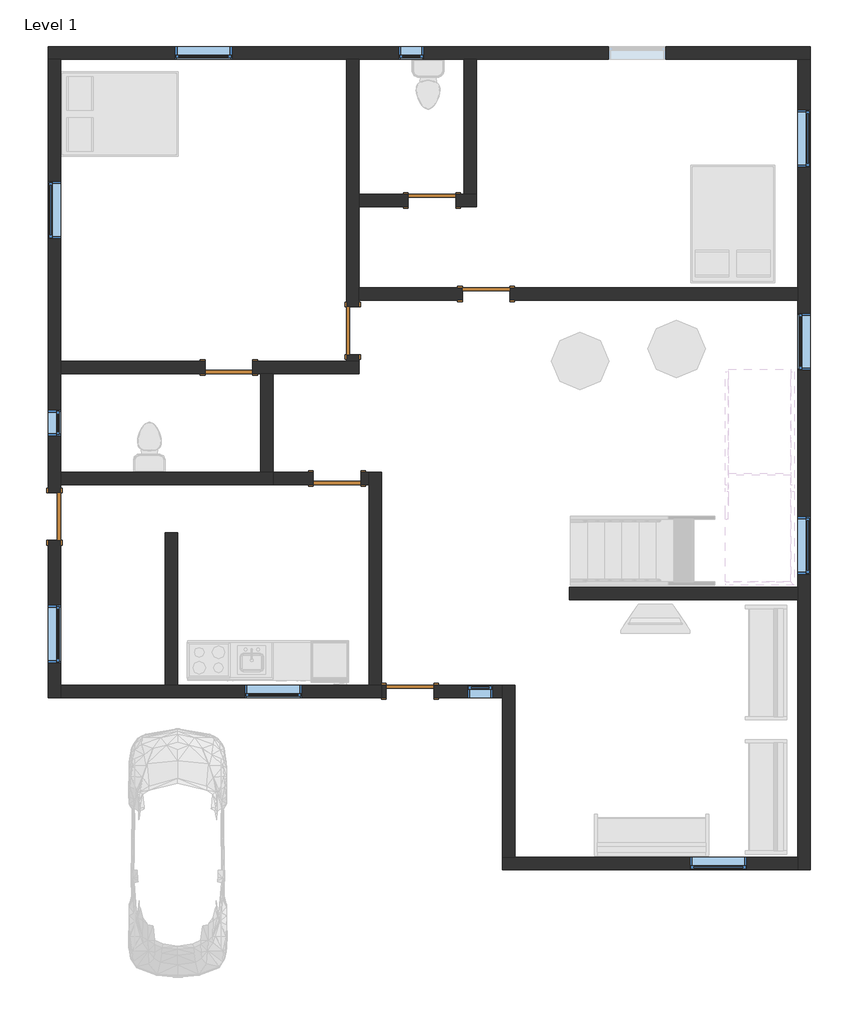
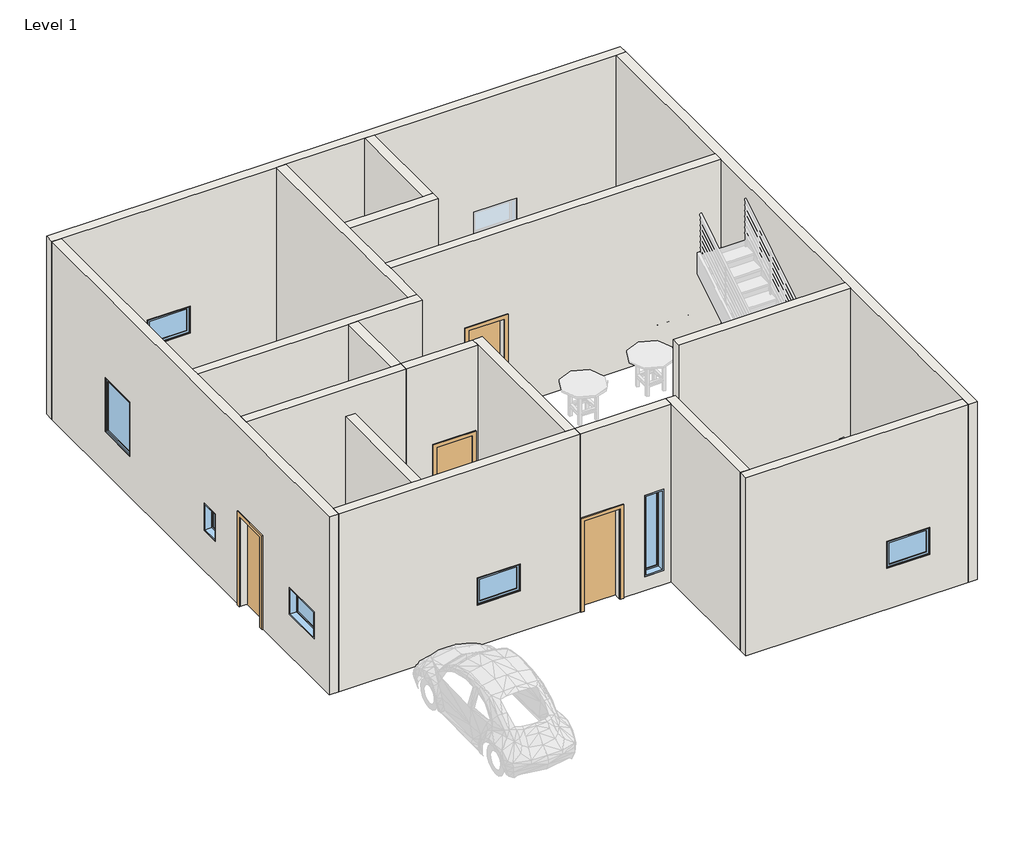
# One storey, part 1 of 4: 18 walls, 11 windows, 7 doors.
"""IFC4 building model written with IfcOpenShell, lengths in millimetres."""

from ifc_helpers import new_model, si_unit, frame, origin, origin_with_axes, place, context, project, spatial, polyline, outline, extrude, faceted_brep, transform, mapped, element, save
from components import m_single_flush_0762_x_2032mm_0c256fab, m_single_flush_0762_x_2032mm_7341a4fb, m_fixed_0406_x_0610mm_8205b201, m_fixed_0406_x_1830mm_fda39e01, m_fixed_0915_x_0610mm_70a843a6, m_fixed_0915_x_1220mm_488fb2fb

model = new_model("IFC4")

# Units and contexts
model_context = context("Model", 3, world=origin())
ifc_project = project(units=[si_unit("LENGTHUNIT", "METRE", prefix="MILLI")], contexts=[model_context])

# Site, building, storey
site = spatial("IfcSite", under=ifc_project)
building = spatial("IfcBuilding", under=site)
storey = spatial("IfcBuildingStorey", under=building, Name="Level 1", Elevation=0.0)

# Doors
placement = place(None, origin())
m_single_flush_0762_x_2032mm_shape = m_single_flush_0762_x_2032mm_0c256fab(model_context)
element("IfcDoor", 1, ObjectType="M_Single-Flush : 0762 x 2032mm", at=placement, inside=storey, context=model_context, shape_type="MappedRepresentation", body=[
    mapped(m_single_flush_0762_x_2032mm_shape, transform((-2615.9732634, 8846.648464, 0.0), x_axis=(1.0, 0.0, 0.0), y_axis=(0.0, 1.0, 0.0), z_axis=(0.0, 0.0, 1.0))),
])
m_single_flush_0762_x_2032mm_2_shape = m_single_flush_0762_x_2032mm_7341a4fb(model_context)
element("IfcDoor", 2, ObjectType="M_Single-Flush : 0762 x 2032mm", at=placement, inside=storey, context=model_context, shape_type="MappedRepresentation", body=[
    mapped(m_single_flush_0762_x_2032mm_2_shape, transform((-3882.7732634, 6763.448464, 0.0), x_axis=(0.0, -1.0, 0.0), y_axis=(1.0, 0.0, 0.0), z_axis=(0.0, 0.0, 1.0))),
])
element("IfcDoor", 3, ObjectType="M_Single-Flush : 0762 x 2032mm", at=placement, inside=storey, context=model_context, shape_type="MappedRepresentation", body=[
    mapped(m_single_flush_0762_x_2032mm_2_shape, transform((-1749.1732634, 7349.648464, 0.0), x_axis=(-1.0, 0.0, 0.0), y_axis=(0.0, -1.0, 0.0), z_axis=(0.0, 0.0, 1.0))),
])
element("IfcDoor", 4, ObjectType="M_Single-Flush : 0762 x 2032mm", at=placement, inside=storey, context=model_context, shape_type="MappedRepresentation", body=[
    mapped(m_single_flush_0762_x_2032mm_2_shape, transform((-5863.9732634, 6177.248464, 0.0), x_axis=(1.0, 0.0, 0.0), y_axis=(0.0, 1.0, 0.0), z_axis=(0.0, 0.0, 1.0))),
])
element("IfcDoor", 5, ObjectType="M_Single-Flush : 0762 x 2032mm", at=placement, inside=storey, context=model_context, shape_type="MappedRepresentation", body=[
    mapped(m_single_flush_0762_x_2032mm_2_shape, transform((-4132.0232634, 4402.448464, 0.0), x_axis=(1.0, 0.0, 0.0), y_axis=(0.0, 1.0, 0.0), z_axis=(0.0, 0.0, 1.0))),
])
element("IfcDoor", 6, ObjectType="M_Single-Flush : 0762 x 2032mm", at=placement, inside=storey, context=model_context, shape_type="MappedRepresentation", body=[
    mapped(m_single_flush_0762_x_2032mm_2_shape, transform((-8654.7732634, 3791.248464, 0.0), x_axis=(0.0, 1.0, 0.0), y_axis=(-1.0, 0.0, 0.0), z_axis=(0.0, 0.0, 1.0))),
])
element("IfcDoor", 7, ObjectType="M_Single-Flush : 0762 x 2032mm", at=placement, inside=storey, context=model_context, shape_type="MappedRepresentation", body=[
    mapped(m_single_flush_0762_x_2032mm_2_shape, transform((-2965.2232634, 998.848464, 0.0), x_axis=(-1.0, 0.0, 0.0), y_axis=(0.0, -1.0, 0.0), z_axis=(0.0, 0.0, 1.0))),
])

# Walls
element("IfcWall", 8, ObjectType="Generic - 200mm", at=placement, inside=storey, context=model_context, shape_type="Brep", body=[
    faceted_brep([(-8754.7732634, 11104.848464, 0.0), (-8554.7732634, 11104.848464, 0.0), (-3982.7732634, 11104.848464, 0.0), (-3782.7732634, 11104.848464, 0.0), (-2106.3732634, 11104.848464, 0.0), (-1906.3732634, 11104.848464, 0.0), (3237.2267366, 11104.848464, 0.0), (3437.2267366, 11104.848464, 0.0), (3437.2267366, 11104.848464, 4000.0), (3237.2267366, 11104.848464, 4000.0), (-1906.3732634, 11104.848464, 4000.0), (-2106.3732634, 11104.848464, 4000.0), (-3782.7732634, 11104.848464, 4000.0), (-3982.7732634, 11104.848464, 4000.0), (-8554.7732634, 11104.848464, 4000.0), (-8754.7732634, 11104.848464, 4000.0), (207.9267366, 11104.848464, 915.0), (207.9267366, 11104.848464, 1525.0), (1122.9267366, 11104.848464, 1525.0), (1122.9267366, 11104.848464, 915.0), (-5811.2732634, 11104.848464, 915.0), (-6726.2732634, 11104.848464, 915.0), (-6726.2732634, 11104.848464, 1525.0), (-5811.2732634, 11104.848464, 1525.0), (-2741.5732634, 11104.848464, 915.0), (-3147.5732634, 11104.848464, 915.0), (-3147.5732634, 11104.848464, 1525.0), (-2741.5732634, 11104.848464, 1525.0), (-8754.7732634, 11304.848464, 0.0), (-8754.7732634, 11304.848464, 4000.0), (3437.2267366, 11304.848464, 4000.0), (3437.2267366, 11304.848464, 0.0), (207.9267366, 11304.848464, 915.0), (1122.9267366, 11304.848464, 915.0), (1122.9267366, 11304.848464, 1525.0), (207.9267366, 11304.848464, 1525.0), (-5811.2732634, 11304.848464, 915.0), (-5811.2732634, 11304.848464, 1525.0), (-6726.2732634, 11304.848464, 1525.0), (-6726.2732634, 11304.848464, 915.0), (-2741.5732634, 11304.848464, 915.0), (-2741.5732634, 11304.848464, 1525.0), (-3147.5732634, 11304.848464, 1525.0), (-3147.5732634, 11304.848464, 915.0)], [[[0, 1, 2, 3, 4, 5, 6, 7, 8, 9, 10, 11, 12, 13, 14, 15], [16, 17, 18, 19], [20, 21, 22, 23], [24, 25, 26, 27]], [[28, 29, 30, 31], [32, 33, 34, 35], [36, 37, 38, 39], [40, 41, 42, 43]], [[7, 6, 5, 4, 3, 2, 1, 0, 28, 31]], [[15, 14, 13, 12, 11, 10, 9, 8, 30, 29]], [[8, 7, 31, 30]], [[0, 15, 29, 28]], [[17, 16, 32, 35]], [[18, 17, 35, 34]], [[19, 18, 34, 33]], [[16, 19, 33, 32]], [[37, 36, 20, 23]], [[38, 37, 23, 22]], [[39, 38, 22, 21]], [[36, 39, 21, 20]], [[41, 40, 24, 27]], [[42, 41, 27, 26]], [[43, 42, 26, 25]], [[40, 43, 25, 24]]]),
])
element("IfcWall", 9, ObjectType="Generic - 200mm", at=placement, inside=storey, context=model_context, shape_type="Brep", body=[
    faceted_brep([(3237.2267366, 11104.848464, 0.0), (3237.2267366, 7449.648464, 0.0), (3237.2267366, 7249.648464, 0.0), (3237.2267366, 2665.698464, 0.0), (3237.2267366, 2465.698464, 0.0), (3237.2267366, -1653.951536, 0.0), (3237.2267366, -1853.951536, 0.0), (3237.2267366, -1853.951536, 4000.0), (3237.2267366, -1653.951536, 4000.0), (3237.2267366, 2465.698464, 4000.0), (3237.2267366, 2665.698464, 4000.0), (3237.2267366, 7249.648464, 4000.0), (3237.2267366, 7449.648464, 4000.0), (3237.2267366, 11104.848464, 4000.0), (3237.2267366, 3785.198464, 915.0), (3237.2267366, 3785.198464, 1525.0), (3237.2267366, 2870.198464, 1525.0), (3237.2267366, 2870.198464, 915.0), (3237.2267366, 6130.148464, 915.0), (3237.2267366, 7045.148464, 915.0), (3237.2267366, 7045.148464, 1525.0), (3237.2267366, 6130.148464, 1525.0), (3237.2267366, 10290.748464, 915.0), (3237.2267366, 10290.748464, 1525.0), (3237.2267366, 9375.748464, 1525.0), (3237.2267366, 9375.748464, 915.0), (3437.2267366, 11104.848464, 0.0), (3437.2267366, 11104.848464, 4000.0), (3437.2267366, -1853.951536, 4000.0), (3437.2267366, -1853.951536, 0.0), (3437.2267366, 3785.198464, 915.0), (3437.2267366, 2870.198464, 915.0), (3437.2267366, 2870.198464, 1525.0), (3437.2267366, 3785.198464, 1525.0), (3437.2267366, 6130.148464, 915.0), (3437.2267366, 6130.148464, 1525.0), (3437.2267366, 7045.148464, 1525.0), (3437.2267366, 7045.148464, 915.0), (3437.2267366, 10290.748464, 915.0), (3437.2267366, 9375.748464, 915.0), (3437.2267366, 9375.748464, 1525.0), (3437.2267366, 10290.748464, 1525.0)], [[[0, 1, 2, 3, 4, 5, 6, 7, 8, 9, 10, 11, 12, 13], [14, 15, 16, 17], [18, 19, 20, 21], [22, 23, 24, 25]], [[26, 27, 28, 29], [30, 31, 32, 33], [34, 35, 36, 37], [38, 39, 40, 41]], [[6, 5, 4, 3, 2, 1, 0, 26, 29]], [[13, 12, 11, 10, 9, 8, 7, 28, 27]], [[0, 13, 27, 26]], [[7, 6, 29, 28]], [[15, 14, 30, 33]], [[16, 15, 33, 32]], [[17, 16, 32, 31]], [[14, 17, 31, 30]], [[35, 34, 18, 21]], [[36, 35, 21, 20]], [[37, 36, 20, 19]], [[34, 37, 19, 18]], [[23, 22, 38, 41]], [[24, 23, 41, 40]], [[25, 24, 40, 39]], [[22, 25, 39, 38]]]),
])
element("IfcWall", 10, ObjectType="Generic - 200mm", at=placement, inside=storey, context=model_context, shape_type="Brep", body=[
    faceted_brep([(-8554.7732634, 4172.248464, 2032.0), (-8554.7732634, 4172.248464, 0.0), (-8554.7732634, 4300.848464, 0.0), (-8554.7732634, 4500.848464, 0.0), (-8554.7732634, 6077.248464, 0.0), (-8554.7732634, 6277.248464, 0.0), (-8554.7732634, 11104.848464, 0.0), (-8554.7732634, 11104.848464, 4000.0), (-8554.7732634, 6277.248464, 4000.0), (-8554.7732634, 6077.248464, 4000.0), (-8554.7732634, 4500.848464, 4000.0), (-8554.7732634, 4300.848464, 4000.0), (-8554.7732634, 1098.848464, 4000.0), (-8554.7732634, 898.848464, 4000.0), (-8554.7732634, 898.848464, 0.0), (-8554.7732634, 1098.848464, 0.0), (-8554.7732634, 3410.248464, 0.0), (-8554.7732634, 3410.248464, 2032.0), (-8554.7732634, 2370.748464, 915.0), (-8554.7732634, 1455.748464, 915.0), (-8554.7732634, 1455.748464, 1525.0), (-8554.7732634, 2370.748464, 1525.0), (-8554.7732634, 5492.048464, 915.0), (-8554.7732634, 5086.048464, 915.0), (-8554.7732634, 5086.048464, 1525.0), (-8554.7732634, 5492.048464, 1525.0), (-8554.7732634, 8233.548464, 915.0), (-8554.7732634, 8233.548464, 2135.0), (-8554.7732634, 9148.548464, 2135.0), (-8554.7732634, 9148.548464, 915.0), (-8754.7732634, 11104.848464, 0.0), (-8754.7732634, 4172.248464, 0.0), (-8754.7732634, 4172.248464, 2032.0), (-8754.7732634, 3410.248464, 2032.0), (-8754.7732634, 3410.248464, 0.0), (-8754.7732634, 898.848464, 0.0), (-8754.7732634, 898.848464, 4000.0), (-8754.7732634, 11104.848464, 4000.0), (-8754.7732634, 2370.748464, 915.0), (-8754.7732634, 2370.748464, 1525.0), (-8754.7732634, 1455.748464, 1525.0), (-8754.7732634, 1455.748464, 915.0), (-8754.7732634, 5492.048464, 915.0), (-8754.7732634, 5492.048464, 1525.0), (-8754.7732634, 5086.048464, 1525.0), (-8754.7732634, 5086.048464, 915.0), (-8754.7732634, 8233.548464, 915.0), (-8754.7732634, 9148.548464, 915.0), (-8754.7732634, 9148.548464, 2135.0), (-8754.7732634, 8233.548464, 2135.0)], [[[0, 1, 2, 3, 4, 5, 6, 7, 8, 9, 10, 11, 12, 13, 14, 15, 16, 17], [18, 19, 20, 21], [22, 23, 24, 25], [26, 27, 28, 29]], [[30, 31, 32, 33, 34, 35, 36, 37], [38, 39, 40, 41], [42, 43, 44, 45], [46, 47, 48, 49]], [[6, 5, 4, 3, 2, 1, 31, 30]], [[16, 15, 14, 35, 34]], [[13, 12, 11, 10, 9, 8, 7, 37, 36]], [[7, 6, 30, 37]], [[32, 31, 1, 0]], [[33, 32, 0, 17]], [[34, 33, 17, 16]], [[14, 13, 36, 35]], [[39, 38, 18, 21]], [[40, 39, 21, 20]], [[41, 40, 20, 19]], [[38, 41, 19, 18]], [[43, 42, 22, 25]], [[44, 43, 25, 24]], [[45, 44, 24, 23]], [[42, 45, 23, 22]], [[27, 26, 46, 49]], [[28, 27, 49, 48]], [[29, 28, 48, 47]], [[26, 29, 47, 46]]]),
])
element("IfcWall", 11, ObjectType="Generic - 200mm", at=placement, inside=storey, context=model_context, shape_type="Brep", body=[
    faceted_brep([(-5482.9732634, 6077.248464, 2032.0), (-5482.9732634, 6077.248464, 0.0), (-5354.3732634, 6077.248464, 0.0), (-5154.3732634, 6077.248464, 0.0), (-3782.7732634, 6077.248464, 0.0), (-3782.7732634, 6077.248464, 4000.0), (-5154.3732634, 6077.248464, 4000.0), (-5354.3732634, 6077.248464, 4000.0), (-8554.7732634, 6077.248464, 4000.0), (-8554.7732634, 6077.248464, 0.0), (-6244.9732634, 6077.248464, 0.0), (-6244.9732634, 6077.248464, 2032.0), (-3782.7732634, 6277.248464, 0.0), (-3982.7732634, 6277.248464, 0.0), (-5482.9732634, 6277.248464, 0.0), (-5482.9732634, 6277.248464, 2032.0), (-6244.9732634, 6277.248464, 2032.0), (-6244.9732634, 6277.248464, 0.0), (-8554.7732634, 6277.248464, 0.0), (-8554.7732634, 6277.248464, 4000.0), (-3982.7732634, 6277.248464, 4000.0), (-3782.7732634, 6277.248464, 4000.0)], [[[0, 1, 2, 3, 4, 5, 6, 7, 8, 9, 10, 11]], [[12, 13, 14, 15, 16, 17, 18, 19, 20, 21]], [[10, 9, 18, 17]], [[4, 3, 2, 1, 14, 13, 12]], [[8, 7, 6, 5, 21, 20, 19]], [[9, 8, 19, 18]], [[5, 4, 12, 21]], [[15, 14, 1, 0]], [[16, 15, 0, 11]], [[17, 16, 11, 10]]]),
])
element("IfcWall", 12, ObjectType="Generic - 200mm", at=placement, inside=storey, context=model_context, shape_type="Brep", body=[
    faceted_brep([(-3782.7732634, 6277.248464, 0.0), (-3782.7732634, 6382.448464, 0.0), (-3782.7732634, 6382.448464, 2032.0), (-3782.7732634, 7144.448464, 2032.0), (-3782.7732634, 7144.448464, 0.0), (-3782.7732634, 7249.648464, 0.0), (-3782.7732634, 7449.648464, 0.0), (-3782.7732634, 8746.648464, 0.0), (-3782.7732634, 8946.648464, 0.0), (-3782.7732634, 11104.848464, 0.0), (-3782.7732634, 11104.848464, 4000.0), (-3782.7732634, 8946.648464, 4000.0), (-3782.7732634, 8746.648464, 4000.0), (-3782.7732634, 7449.648464, 4000.0), (-3782.7732634, 7249.648464, 4000.0), (-3782.7732634, 6277.248464, 4000.0), (-3982.7732634, 6382.448464, 2032.0), (-3982.7732634, 6382.448464, 0.0), (-3982.7732634, 6277.248464, 0.0), (-3982.7732634, 6277.248464, 4000.0), (-3982.7732634, 11104.848464, 4000.0), (-3982.7732634, 11104.848464, 0.0), (-3982.7732634, 7144.448464, 0.0), (-3982.7732634, 7144.448464, 2032.0)], [[[0, 1, 2, 3, 4, 5, 6, 7, 8, 9, 10, 11, 12, 13, 14, 15]], [[16, 17, 18, 19, 20, 21, 22, 23]], [[22, 21, 9, 8, 7, 6, 5, 4]], [[18, 17, 1, 0]], [[15, 14, 13, 12, 11, 10, 20, 19]], [[0, 15, 19, 18]], [[10, 9, 21, 20]], [[2, 1, 17, 16]], [[3, 2, 16, 23]], [[4, 3, 23, 22]]]),
])
element("IfcWall", 13, ObjectType="Generic - 200mm", at=placement, inside=storey, context=model_context, shape_type="Brep", body=[
    faceted_brep([(-2234.9732634, 8746.648464, 2032.0), (-2234.9732634, 8746.648464, 0.0), (-1906.3732634, 8746.648464, 0.0), (-1906.3732634, 8746.648464, 4000.0), (-3782.7732634, 8746.648464, 4000.0), (-3782.7732634, 8746.648464, 0.0), (-2996.9732634, 8746.648464, 0.0), (-2996.9732634, 8746.648464, 2032.0), (-1906.3732634, 8946.648464, 0.0), (-2106.3732634, 8946.648464, 0.0), (-2234.9732634, 8946.648464, 0.0), (-2234.9732634, 8946.648464, 2032.0), (-2996.9732634, 8946.648464, 2032.0), (-2996.9732634, 8946.648464, 0.0), (-3782.7732634, 8946.648464, 0.0), (-3782.7732634, 8946.648464, 4000.0), (-2106.3732634, 8946.648464, 4000.0), (-1906.3732634, 8946.648464, 4000.0)], [[[0, 1, 2, 3, 4, 5, 6, 7]], [[8, 9, 10, 11, 12, 13, 14, 15, 16, 17]], [[6, 5, 14, 13]], [[2, 1, 10, 9, 8]], [[4, 3, 17, 16, 15]], [[5, 4, 15, 14]], [[3, 2, 8, 17]], [[11, 10, 1, 0]], [[12, 11, 0, 7]], [[13, 12, 7, 6]]]),
])
element("IfcWall", 14, ObjectType="Generic - 200mm", at=placement, inside=storey, context=model_context, shape_type="SweptSolid", body=[
    extrude(outline(polyline([(-1906.3732634, 11104.848464), (-1906.3732634, 8946.648464), (-2106.3732634, 8946.648464), (-2106.3732634, 11104.848464), (-1906.3732634, 11104.848464)])), origin_with_axes(), (0.0, 0.0, 1.0), 4000.0),
])
element("IfcWall", 15, ObjectType="Generic - 200mm", at=placement, inside=storey, context=model_context, shape_type="SweptSolid", body=[
    extrude(outline(polyline([(0.0, -3782.7732634), (0.0, -2130.1732634), (2032.0, -2130.1732634), (2032.0, -1368.1732634), (0.0, -1368.1732634), (0.0, 3237.2267366), (4000.0, 3237.2267366), (4000.0, -3782.7732634), (0.0, -3782.7732634)])), frame((0.0, 7249.648464, 0.0), z_axis=(0.0, 1.0, 0.0), x_axis=(0.0, 0.0, 1.0)), (0.0, 0.0, 1.0), 200.0),
])
element("IfcWall", 16, ObjectType="Generic - 200mm", at=placement, inside=storey, context=model_context, shape_type="Brep", body=[
    faceted_brep([(-8554.7732634, 4300.848464, 0.0), (-5154.3732634, 4300.848464, 0.0), (-5154.3732634, 4300.848464, 4000.0), (-8554.7732634, 4300.848464, 4000.0), (-8554.7732634, 4500.848464, 0.0), (-8554.7732634, 4500.848464, 4000.0), (-5354.3732634, 4500.848464, 4000.0), (-5154.3732634, 4500.848464, 4000.0), (-5154.3732634, 4500.848464, 0.0), (-5354.3732634, 4500.848464, 0.0), (-5154.3732634, 4302.448464, 0.0), (-5154.3732634, 4302.448464, 4000.0)], [[[0, 1, 2, 3]], [[4, 5, 6, 7, 8, 9]], [[1, 0, 4, 9, 8, 10]], [[3, 2, 11, 7, 6, 5]], [[0, 3, 5, 4]], [[2, 1, 10, 8, 7, 11]]]),
])
element("IfcWall", 17, ObjectType="Generic - 200mm", at=placement, inside=storey, context=model_context, shape_type="Brep", body=[
    faceted_brep([(-5154.3732634, 4500.848464, 0.0), (-5154.3732634, 4502.448464, 0.0), (-5154.3732634, 6077.248464, 0.0), (-5154.3732634, 6077.248464, 4000.0), (-5154.3732634, 4502.448464, 4000.0), (-5154.3732634, 4500.848464, 4000.0), (-5354.3732634, 4500.848464, 0.0), (-5354.3732634, 4500.848464, 4000.0), (-5354.3732634, 6077.248464, 4000.0), (-5354.3732634, 6077.248464, 0.0)], [[[0, 1, 2, 3, 4, 5]], [[6, 7, 8, 9]], [[2, 1, 0, 6, 9]], [[5, 4, 3, 8, 7]], [[0, 5, 7, 6]], [[3, 2, 9, 8]]]),
])
element("IfcWall", 18, ObjectType="Generic - 200mm", at=placement, inside=storey, context=model_context, shape_type="Brep", body=[
    faceted_brep([(-8554.7732634, 898.848464, 0.0), (-3422.4232634, 898.848464, 0.0), (-3422.4232634, 898.848464, 4000.0), (-8554.7732634, 898.848464, 4000.0), (-4693.6982634, 898.848464, 915.0), (-5608.6982634, 898.848464, 915.0), (-5608.6982634, 898.848464, 1525.0), (-4693.6982634, 898.848464, 1525.0), (-8554.7732634, 1098.848464, 0.0), (-8554.7732634, 1098.848464, 4000.0), (-6879.9732634, 1098.848464, 4000.0), (-6679.9732634, 1098.848464, 4000.0), (-3622.4232634, 1098.848464, 4000.0), (-3422.4232634, 1098.848464, 4000.0), (-3422.4232634, 1098.848464, 0.0), (-3622.4232634, 1098.848464, 0.0), (-6679.9732634, 1098.848464, 0.0), (-6879.9732634, 1098.848464, 0.0), (-4693.6982634, 1098.848464, 915.0), (-4693.6982634, 1098.848464, 1525.0), (-5608.6982634, 1098.848464, 1525.0), (-5608.6982634, 1098.848464, 915.0)], [[[0, 1, 2, 3], [4, 5, 6, 7]], [[8, 9, 10, 11, 12, 13, 14, 15, 16, 17], [18, 19, 20, 21]], [[1, 0, 8, 17, 16, 15, 14]], [[3, 2, 13, 12, 11, 10, 9]], [[2, 1, 14, 13]], [[0, 3, 9, 8]], [[19, 18, 4, 7]], [[20, 19, 7, 6]], [[21, 20, 6, 5]], [[18, 21, 5, 4]]]),
])
element("IfcWall", 19, ObjectType="Generic - 200mm", at=placement, inside=storey, context=model_context, shape_type="SweptSolid", body=[
    extrude(outline(polyline([(-6679.9732634, 3537.248464), (-6679.9732634, 1098.848464), (-6879.9732634, 1098.848464), (-6879.9732634, 3537.248464), (-6679.9732634, 3537.248464)])), origin_with_axes(), (0.0, 0.0, 1.0), 4000.0),
])
element("IfcWall", 20, ObjectType="Generic - 200mm", at=placement, inside=storey, context=model_context, shape_type="Brep", body=[
    faceted_brep([(-3422.4232634, 1098.848464, 0.0), (-3422.4232634, 4502.448464, 0.0), (-3422.4232634, 4502.448464, 4000.0), (-3422.4232634, 1098.848464, 4000.0), (-3622.4232634, 1098.848464, 0.0), (-3622.4232634, 1098.848464, 4000.0), (-3622.4232634, 4302.448464, 4000.0), (-3622.4232634, 4502.448464, 4000.0), (-3622.4232634, 4502.448464, 0.0), (-3622.4232634, 4302.448464, 0.0)], [[[0, 1, 2, 3]], [[4, 5, 6, 7, 8, 9]], [[1, 0, 4, 9, 8]], [[3, 2, 7, 6, 5]], [[0, 3, 5, 4]], [[2, 1, 8, 7]]]),
])
element("IfcWall", 21, ObjectType="Generic - 200mm", at=placement, inside=storey, context=model_context, shape_type="Brep", body=[
    faceted_brep([(-3622.4232634, 4502.448464, 0.0), (-3751.0232634, 4502.448464, 0.0), (-3751.0232634, 4502.448464, 2032.0), (-4513.0232634, 4502.448464, 2032.0), (-4513.0232634, 4502.448464, 0.0), (-5154.3732634, 4502.448464, 0.0), (-5154.3732634, 4502.448464, 4000.0), (-3622.4232634, 4502.448464, 4000.0), (-3751.0232634, 4302.448464, 2032.0), (-3751.0232634, 4302.448464, 0.0), (-3622.4232634, 4302.448464, 0.0), (-3622.4232634, 4302.448464, 4000.0), (-5154.3732634, 4302.448464, 4000.0), (-5154.3732634, 4302.448464, 0.0), (-4513.0232634, 4302.448464, 0.0), (-4513.0232634, 4302.448464, 2032.0), (-5154.3732634, 4500.848464, 0.0), (-5154.3732634, 4500.848464, 4000.0)], [[[0, 1, 2, 3, 4, 5, 6, 7]], [[8, 9, 10, 11, 12, 13, 14, 15]], [[14, 13, 16, 5, 4]], [[10, 9, 1, 0]], [[7, 6, 17, 12, 11]], [[6, 5, 16, 13, 12, 17]], [[0, 7, 11, 10]], [[2, 1, 9, 8]], [[3, 2, 8, 15]], [[4, 3, 15, 14]]]),
])
element("IfcWall", 22, ObjectType="Generic - 200mm", at=placement, inside=storey, context=model_context, shape_type="SweptSolid", body=[
    extrude(outline(polyline([(-420.3732634, 2665.698464), (3237.2267366, 2665.698464), (3237.2267366, 2465.698464), (-420.3732634, 2465.698464), (-420.3732634, 2665.698464)])), origin_with_axes(), (0.0, 0.0, 1.0), 4000.0),
])
element("IfcWall", 23, ObjectType="Generic - 200mm", at=placement, inside=storey, context=model_context, shape_type="Brep", body=[
    faceted_brep([(3237.2267366, -1653.951536, 0.0), (-1287.1732634, -1653.951536, 0.0), (-1487.1732634, -1653.951536, 0.0), (-1487.1732634, -1653.951536, 4000.0), (-1287.1732634, -1653.951536, 4000.0), (3237.2267366, -1653.951536, 4000.0), (2423.1267366, -1653.951536, 915.0), (2423.1267366, -1653.951536, 1525.0), (1508.1267366, -1653.951536, 1525.0), (1508.1267366, -1653.951536, 915.0), (3237.2267366, -1853.951536, 0.0), (3237.2267366, -1853.951536, 4000.0), (-1487.1732634, -1853.951536, 4000.0), (-1487.1732634, -1853.951536, 0.0), (2423.1267366, -1853.951536, 915.0), (1508.1267366, -1853.951536, 915.0), (1508.1267366, -1853.951536, 1525.0), (2423.1267366, -1853.951536, 1525.0)], [[[0, 1, 2, 3, 4, 5], [6, 7, 8, 9]], [[10, 11, 12, 13], [14, 15, 16, 17]], [[2, 1, 0, 10, 13]], [[5, 4, 3, 12, 11]], [[3, 2, 13, 12]], [[0, 5, 11, 10]], [[7, 6, 14, 17]], [[8, 7, 17, 16]], [[9, 8, 16, 15]], [[6, 9, 15, 14]]]),
])
element("IfcWall", 24, ObjectType="Generic - 200mm", at=placement, inside=storey, context=model_context, shape_type="Brep", body=[
    faceted_brep([(-1287.1732634, -1653.951536, 0.0), (-1287.1732634, 1098.848464, 0.0), (-1287.1732634, 1098.848464, 4000.0), (-1287.1732634, -1653.951536, 4000.0), (-1487.1732634, -1653.951536, 0.0), (-1487.1732634, -1653.951536, 4000.0), (-1487.1732634, 898.848464, 4000.0), (-1487.1732634, 1098.848464, 4000.0), (-1487.1732634, 1098.848464, 0.0), (-1487.1732634, 898.848464, 0.0)], [[[0, 1, 2, 3]], [[4, 5, 6, 7, 8, 9]], [[1, 0, 4, 9, 8]], [[3, 2, 7, 6, 5]], [[0, 3, 5, 4]], [[2, 1, 8, 7]]]),
])
element("IfcWall", 25, ObjectType="Generic - 200mm", at=placement, inside=storey, context=model_context, shape_type="SweptSolid", body=[
    extrude(outline(polyline([(0.0, -3422.4232634), (0.0, -3346.2232634), (2032.0, -3346.2232634), (2032.0, -2584.2232634), (0.0, -2584.2232634), (0.0, -1487.1732634), (4000.0, -1487.1732634), (4000.0, -3422.4232634), (0.0, -3422.4232634)]), holes=[polyline([(305.0, -2047.3732634), (2135.0, -2047.3732634), (2135.0, -1641.3732634), (305.0, -1641.3732634), (305.0, -2047.3732634)])]), frame((0.0, 898.848464, 0.0), z_axis=(0.0, 1.0, 0.0), x_axis=(0.0, 0.0, 1.0)), (0.0, 0.0, 1.0), 200.0),
])

# Windows
m_fixed_0406_x_0610mm_shape = m_fixed_0406_x_0610mm_8205b201(model_context)
element("IfcWindow", 26, ObjectType="M_Fixed : 0406 x 0610mm", at=placement, inside=storey, context=model_context, shape_type="MappedRepresentation", body=[
    mapped(m_fixed_0406_x_0610mm_shape, transform((-2944.5732634, 11217.848464, 0.0), x_axis=(-1.0, 0.0, 0.0), y_axis=(0.0, -1.0, 0.0), z_axis=(0.0, 0.0, 1.0))),
])
element("IfcWindow", 27, ObjectType="M_Fixed : 0406 x 0610mm", at=placement, inside=storey, context=model_context, shape_type="MappedRepresentation", body=[
    mapped(m_fixed_0406_x_0610mm_shape, transform((-8667.7732634, 5289.048464, 0.0), x_axis=(0.0, -1.0, 0.0), y_axis=(1.0, 0.0, 0.0), z_axis=(0.0, 0.0, 1.0))),
])
m_fixed_0406_x_1830mm_shape = m_fixed_0406_x_1830mm_fda39e01(model_context)
element("IfcWindow", 28, ObjectType="M_Fixed : 0406 x 1830mm", at=placement, inside=storey, context=model_context, shape_type="MappedRepresentation", body=[
    mapped(m_fixed_0406_x_1830mm_shape, transform((-1844.3732634, 985.848464, 0.0), x_axis=(1.0, 0.0, 0.0), y_axis=(0.0, 1.0, 0.0), z_axis=(0.0, 0.0, 1.0))),
])
m_fixed_0915_x_0610mm_shape = m_fixed_0915_x_0610mm_70a843a6(model_context)
element("IfcWindow", 29, ObjectType="M_Fixed : 0915 x 0610mm", at=placement, inside=storey, context=model_context, shape_type="MappedRepresentation", body=[
    mapped(m_fixed_0915_x_0610mm_shape, transform((-8667.7732634, 1913.248464, 0.0), x_axis=(0.0, -1.0, 0.0), y_axis=(1.0, 0.0, 0.0), z_axis=(0.0, 0.0, 1.0))),
])
element("IfcWindow", 30, ObjectType="M_Fixed : 0915 x 0610mm", at=placement, inside=storey, context=model_context, shape_type="MappedRepresentation", body=[
    mapped(m_fixed_0915_x_0610mm_shape, transform((-5151.1982634, 1011.848464, 0.0), x_axis=(-1.0, 0.0, 0.0), y_axis=(0.0, -1.0, 0.0), z_axis=(0.0, 0.0, 1.0))),
])
element("IfcWindow", 31, ObjectType="M_Fixed : 0915 x 0610mm", at=placement, inside=storey, context=model_context, shape_type="MappedRepresentation", body=[
    mapped(m_fixed_0915_x_0610mm_shape, transform((1965.6267366, -1740.951536, 0.0), x_axis=(-1.0, 0.0, 0.0), y_axis=(0.0, -1.0, 0.0), z_axis=(0.0, 0.0, 1.0))),
])
element("IfcWindow", 32, ObjectType="M_Fixed : 0915 x 0610mm", at=placement, inside=storey, context=model_context, shape_type="MappedRepresentation", body=[
    mapped(m_fixed_0915_x_0610mm_shape, transform((3324.2267366, 3327.698464, 0.0), x_axis=(0.0, -1.0, 0.0), y_axis=(1.0, 0.0, 0.0), z_axis=(0.0, 0.0, 1.0))),
])
element("IfcWindow", 33, ObjectType="M_Fixed : 0915 x 0610mm", at=placement, inside=storey, context=model_context, shape_type="MappedRepresentation", body=[
    mapped(m_fixed_0915_x_0610mm_shape, transform((3350.2267366, 6587.648464, 0.0), x_axis=(0.0, 1.0, 0.0), y_axis=(-1.0, 0.0, 0.0), z_axis=(0.0, 0.0, 1.0))),
])
element("IfcWindow", 34, ObjectType="M_Fixed : 0915 x 0610mm", at=placement, inside=storey, context=model_context, shape_type="MappedRepresentation", body=[
    mapped(m_fixed_0915_x_0610mm_shape, transform((3324.2267366, 9833.248464, 0.0), x_axis=(0.0, -1.0, 0.0), y_axis=(1.0, 0.0, 0.0), z_axis=(0.0, 0.0, 1.0))),
])
element("IfcWindow", 35, ObjectType="M_Fixed : 0915 x 0610mm", at=placement, inside=storey, context=model_context, shape_type="MappedRepresentation", body=[
    mapped(m_fixed_0915_x_0610mm_shape, transform((-6268.7732634, 11217.848464, 0.0), x_axis=(-1.0, 0.0, 0.0), y_axis=(0.0, -1.0, 0.0), z_axis=(0.0, 0.0, 1.0))),
])
m_fixed_0915_x_1220mm_shape = m_fixed_0915_x_1220mm_488fb2fb(model_context)
element("IfcWindow", 36, ObjectType="M_Fixed : 0915 x 1220mm", at=placement, inside=storey, context=model_context, shape_type="MappedRepresentation", body=[
    mapped(m_fixed_0915_x_1220mm_shape, transform((-8641.7732634, 8691.048464, 0.0), x_axis=(0.0, 1.0, 0.0), y_axis=(-1.0, 0.0, 0.0), z_axis=(0.0, 0.0, 1.0))),
])

save(model, "model.ifc")

# Revit data of these elements
# Type "M_Single-Flush : 0762 x 2032mm"
#   Type Mark = "19"
#   Thickness = 0' - 2.00787"
#   Height = 6' - 8"
#   Trim Projection Ext = 0' - 0.98425"
#   Trim Projection Int = 0' - 0.98425"
#   Trim Width = 0' - 2.99213"
#   Width = 2' - 6"
#   Door Material = Door - Panel
#   Frame Material = Door - Frame
#   Function = (empty or 0)
#   Wall Closure = (empty or 0)
# Type "Generic - 200mm"
#   Layers, outside or top first: 0' - 7.87402" no material (function 1)
# Type "M_Fixed : 0406 x 0610mm"
#   Type Mark = "10"
#   Height = 2' - 0.01575"
#   Default Sill Height = 3' - 0.02362"
#   Width = 1' - 3.98425"
#   Window Inset = 0' - 0.74803"
#   Frame Exterior Material = Sash
#   Frame Interior Material = Sash
#   Glass Pane Material = Glass
#   Sash = Sash
#   Wall Closure = (empty or 0)
# Type "M_Fixed : 0406 x 1830mm"
#   Type Mark = "16"
#   Height = 6' - 0.04724"
#   Default Sill Height = 1' - 0.00787"
#   Width = 1' - 3.98425"
#   Window Inset = 0' - 0.74803"
#   Frame Exterior Material = Sash
#   Frame Interior Material = Sash
#   Glass Pane Material = Glass
#   Sash = Sash
#   Wall Closure = (empty or 0)
# Type "M_Fixed : 0915 x 0610mm"
#   Type Mark = "14"
#   Height = 2' - 0.01575"
#   Default Sill Height = 3' - 0.02362"
#   Width = 3' - 0.02362"
#   Window Inset = 0' - 0.74803"
#   Frame Exterior Material = Sash
#   Frame Interior Material = Sash
#   Glass Pane Material = Glass
#   Sash = Sash
#   Wall Closure = (empty or 0)
# Type "M_Fixed : 0915 x 1220mm"
#   Type Mark = "15"
#   Height = 4' - 0.0315"
#   Default Sill Height = 3' - 0.02362"
#   Width = 3' - 0.02362"
#   Window Inset = 0' - 0.74803"
#   Frame Exterior Material = Sash
#   Frame Interior Material = Sash
#   Glass Pane Material = Glass
#   Sash = Sash
#   Wall Closure = (empty or 0)
# Elements 1, 2, 3, 4, 5, 6, 7 (IfcDoor, "M_Single-Flush : 0762 x 2032mm")
#   Phase Created = New Construction
#   Materials on its faces: "Door - Frame", "Door - Panel"
# Elements 8, 9, 10, 11, 12, 13, 14, 15, 16, 17, 18, 19, 20, 21, 22, 23, 24, 25 (IfcWall, "Generic - 200mm")
#   Top Offset = 0' - 0"
#   Base Offset = 0' - 0"
#   wall height = 13' - 1.48031"
#   Phase Created = New Construction
#   Base Constraint = Level 1
#   Top Constraint = Level 2
#   Materials on its faces: "Default Wall"
# Element 26 (IfcWindow, "M_Fixed : 0406 x 0610mm")
#   Mark = "14"
#   Phase Created = New Construction
#   Materials on its faces: "Sash", "Glass"
# Element 27 (IfcWindow, "M_Fixed : 0406 x 0610mm")
#   Mark = "15"
#   Phase Created = New Construction
#   Materials on its faces: "Sash", "Glass"
# Element 28 (IfcWindow, "M_Fixed : 0406 x 1830mm")
#   Mark = "17"
#   Phase Created = New Construction
#   Materials on its faces: "Sash", "Glass"
# Element 29 (IfcWindow, "M_Fixed : 0915 x 0610mm")
#   Mark = "6"
#   Phase Created = New Construction
#   Materials on its faces: "Sash", "Glass"
# Element 30 (IfcWindow, "M_Fixed : 0915 x 0610mm")
#   Mark = "7"
#   Phase Created = New Construction
#   Materials on its faces: "Sash", "Glass"
# Element 31 (IfcWindow, "M_Fixed : 0915 x 0610mm")
#   Mark = "8"
#   Phase Created = New Construction
#   Materials on its faces: "Sash", "Glass"
# Element 32 (IfcWindow, "M_Fixed : 0915 x 0610mm")
#   Mark = "9"
#   Phase Created = New Construction
#   Materials on its faces: "Sash", "Glass"
# Element 33 (IfcWindow, "M_Fixed : 0915 x 0610mm")
#   Mark = "10"
#   Phase Created = New Construction
#   Materials on its faces: "Sash", "Glass"
# Element 34 (IfcWindow, "M_Fixed : 0915 x 0610mm")
#   Mark = "11"
#   Phase Created = New Construction
#   Materials on its faces: "Sash", "Glass"
# Element 35 (IfcWindow, "M_Fixed : 0915 x 0610mm")
#   Mark = "13"
#   Phase Created = New Construction
#   Materials on its faces: "Sash", "Glass"
# Element 36 (IfcWindow, "M_Fixed : 0915 x 1220mm")
#   Mark = "16"
#   Phase Created = New Construction
#   Materials on its faces: "Sash", "Glass"
# Materials
#   "Door - Panel": class "Wood", colour RGB 114 82 51, transparency 0
#   "Door - Frame": colour RGB 153 76 43, transparency 0
#   "Sash": class "Wood", colour RGB 136 99 55, transparency 0
#   "Glass": class "Glass", colour RGB 218 227 224, transparency 0.85, Description = "Soda Lime Glass", Cost = 0
#   "Default Wall": colour RGB 80 80 80, transparency 0
